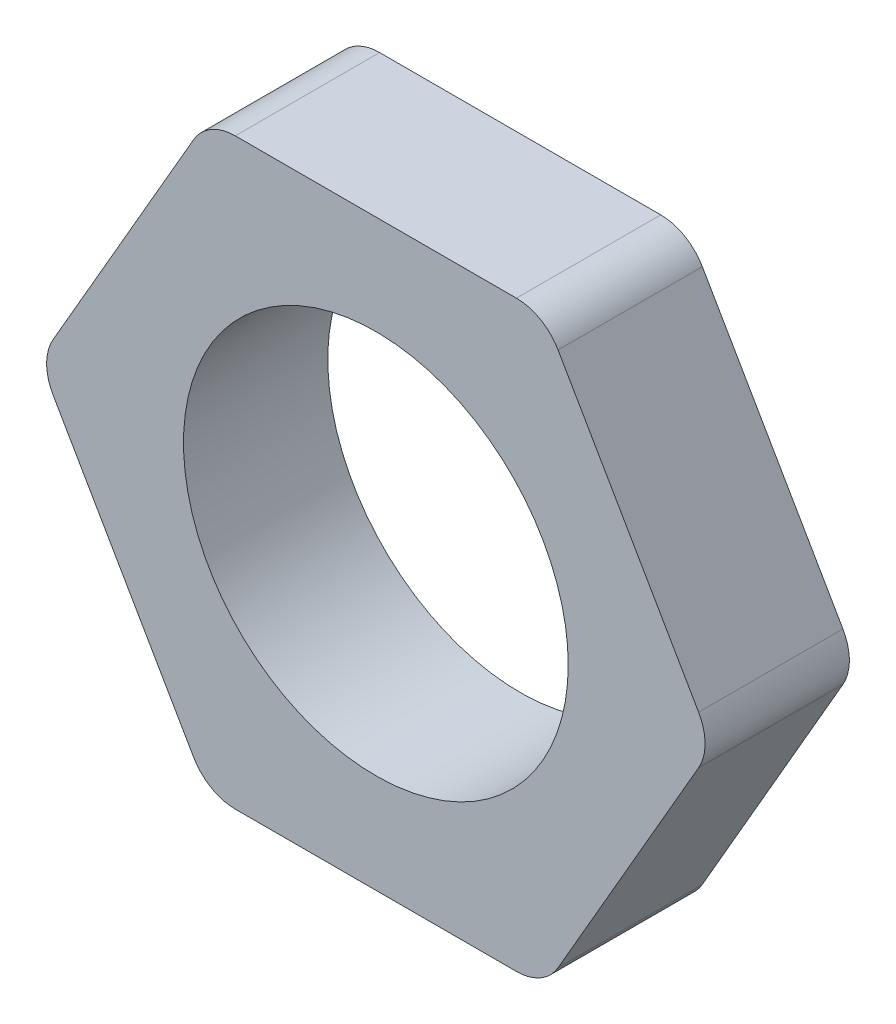
from build123d import *

# Parameters (mm, degrees)
HEX_BODY_DEPTH          = 3
HEX_CORNER_FILLETS_R1_R = 1
BORE_SKETCH_R           = 4
BORE_8_DEPTH            = 3


with BuildPart() as part:
    # Hex Profile Sketch → Hex Body (new body)
    with BuildSketch(Plane.XY):
        Polygon((3.5, -6.062177826), (7, 0), (3.5, 6.062177826), (-3.5, 6.062177826), (-7, 0), (-3.5, -6.062177826), align=None)
    extrude(amount=HEX_BODY_DEPTH)

    # Hex Corner Fillets R1
    hex_corner_fillets_r1_edges = [part.edges().sort_by_distance(p)[0] for p in [
        (-3.5, -6.062177826, 1.5),
        (-7, 0, 1.5),
        (-3.5, 6.062177826, 1.5),
        (3.5, 6.062177826, 1.5),
        (7, 0, 1.5),
        (3.5, -6.062177826, 1.5),
    ]]
    fillet(hex_corner_fillets_r1_edges, radius=HEX_CORNER_FILLETS_R1_R)

    # Bore Sketch → Bore Ø8 (cut)
    with BuildSketch(Plane.XY.offset(3)):
        Circle(BORE_SKETCH_R)
    extrude(amount=-BORE_8_DEPTH, mode=Mode.SUBTRACT)


solid = part.part
